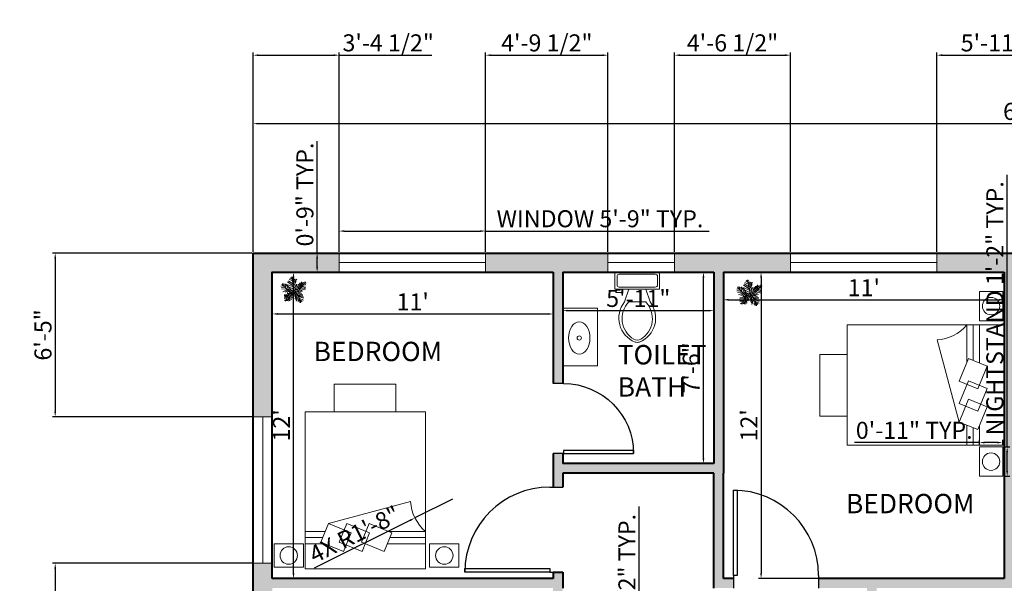
# Model space of a CAD drawing. Units: inches. Extents: x 529 to 1442, y 1029 to 1677.
# Tile 3 of 7: x 529 to 991, y 1412 to 1677. Entities that reach past the tile are written whole.
import ezdxf

# ---------------------------------------------------------------- set-up
doc = ezdxf.new("R2010")
doc.units = ezdxf.units.IN
for name, color, linetype, lineweight in [('A-ANNO-DIMS', 2, 'Continuous', 18), ('A-AREA-IDEN', 7, 'Continuous', 25), ('A-DOOR', 4, 'Continuous', 25), ('A-FLOR-FIXT', 9, 'Continuous', 18), ('A-FURN', 8, 'Continuous', 18), ('A-WALL-PATT', 252, 'Continuous', 13), ('tree', 70, 'Continuous', 13), ('wall', 7, 'Continuous', 40), ('window', 52, 'Continuous', 18)]:
    doc.layers.add(name, color=color, linetype=linetype, lineweight=lineweight)
doc.styles.get("Standard").update_dxf_attribs({"font": 'arial.ttf'})
doc.dimstyles.new('ISO-25', dxfattribs={"dimtxt": 8, "dimasz": 2.5, "dimexe": 1.25, "dimexo": 0.625, "dimtad": 1, "dimdec": 0, "dimlunit": 4, "dimtxsty": 'Standard', "dimcen": 2.5, "dimadec": 0, "dimazin": 0, "dimtfac": 1, "dimtdec": 0, "dimtmove": 0, "dimatfit": 3, "dimfxl": 1, "dimarcsym": 0})

# ---------------------------------------------------------------- blocks, each defined once
blk = doc.blocks.new('*U2')
for p, q in [((0, 0), (0, -6)), ((40, 0), (40, -6))]:
    blk.add_line(p, q)
blk.add_lwpolyline([(0, 0), (0, 40), (1.75, 40), (1.75, 0)], close=True)
blk.add_arc((0, 0), 40, 0, 90)
blk = doc.blocks.new('*U4')
for p, q in [((9.5, -6), (9.5, -2)), ((-10, -8.5), (-8, -8.5)), ((-10, -9.5), (-10, -8.5)), ((-8, -8.5), (-8, -8)), ((-7, -8), (-7, -9.5)), ((-4, -8), (-6, -14)), ((4, -8), (6, -14)), ((-7, -9.5), (-10, -9.5)), ((4, -14), (-4, -14))]:
    blk.add_line(p, q)
blk.add_lwpolyline([(10.5, -8), (10.5, 0), (-10.5, 0), (-10.5, -8)], close=True)
for points in [[(-9.5, -2), (-9.5, -6)], [(8.5, -1), (-8.5, -1)], [(-8.5, -7), (8.5, -7)]]:
    blk.add_lwpolyline(points)
for centre, radius, start, end in [((-8.62, -1.88), 0.884, 81.8699, 188.1301), ((8.62, -1.88), 0.884, 351.8699, 98.1301), ((-8.62, -6.12), 0.884, 171.8699, 278.1301), ((8.62, -6.12), 0.884, 261.8699, 8.1301), ((3.52, -21.58), 12.17, 141.4691, 247.9714), ((4.2, -21.82), 11.33, 136.3677, 238.9468), ((-3.52, -21.58), 12.17, 292.0284, 38.5307), ((-4.2, -21.82), 11.33, 301.053, 43.6321), ((0, -27.88), 4, 245.7318, 294.2682), ((0, -29), 4, 254.8605, 285.1395)]:
    blk.add_arc(centre, radius, start, end)
blk = doc.blocks.new('*U12')
for p, q in [((-7.288, 39.707), (-21.778, 46.673)), ((-8.737, 47.138), (-17.069, 52.711)), ((-10.186, 53.64), (-13.084, 55.962)), ((0, 0), (-10.5, 57)), ((-9.099, 51.782), (-6.563, 55.962)), ((-7.65, 43.423), (-2.578, 49.46)), ((-5.839, 35.992), (4.667, 48.067)), ((-5.114, 27.632), (10.463, 46.673)), ((-47.498, 19.737), (-55.83, 18.344)), ((-40.615, 13.7), (-55.105, 10.913)), ((-31.5, 4.5), (-52.5, 25.5)), ((-33.37, 6.269), (-52.207, 5.34)), ((-48.585, 21.131), (-49.309, 29.026)), ((-28.299, 3.483), (-47.86, -5.805)), ((-43.513, 28.561), (-42.427, 15.558)), ((-38.442, 26.239), (-34.819, 7.663)), ((-21.416, 3.018), (-38.079, -8.128)), ((-35.544, 28.097), (-24.314, 3.947)), ((0, 0), (-31.5, 4.5)), ((-14.533, 2.09), (-30.834, 25.31)), ((-15.982, 2.09), (-30.11, -9.521)), ((-3.665, 19.273), (-27.574, 35.527)), ((-5.114, 28.097), (-24.676, 40.636)), ((-24.314, 23.917), (-2.941, 13.7)), ((0, 0), (-22.5, -19.5)), ((-6.563, 1.161), (-21.416, -8.128)), ((-20.691, 13.7), (-1.129, 4.876)), ((-2.941, 16.486), (8.652, 37.85)), ((-1.129, 6.734), (9.014, 26.704)), ((0, 0), (27, 9)), ((0, 0), (18, -22.5)), ((3.942, 1.625), (11.187, 24.381)), ((6.478, 1.625), (26.04, -8.592)), ((10.101, 3.483), (17.708, 26.239)), ((11.187, 3.483), (30.749, -5.805)), ((16.259, 5.805), (23.142, 31.348)), ((18.07, 5.805), (35.096, -3.483)), ((22.055, 7.198), (27.489, 32.277)), ((24.229, 7.663), (46.688, 1.625)), ((27, 9), (48, 36)), ((27.127, 9.056), (31.112, 35.992)), ((29.662, 12.307), (48.137, 6.269)), ((31.836, 30.883), (32.561, 16.486)), ((33.285, 16.486), (48.862, 10.913)), ((35.096, 32.741), (37.27, 22.524)), ((36.183, 19.737), (48.137, 17.88)), ((38.719, 34.134), (41.979, 28.561)), ((40.53, 25.775), (48.862, 24.846)), ((43.791, 29.954), (51.036, 30.883)), ((44.153, 36.456), (45.239, 32.741)), ((-17.431, -15.094), (-42.789, -18.809)), ((-28.299, -29.026), (-42.789, -31.348)), ((-24.314, -21.596), (-42.427, -22.06)), ((-30.834, -34.135), (-42.427, -35.528)), ((-34.457, -39.708), (-40.978, -42.494)), ((-26.849, -26.24), (-40.253, -25.775)), ((-22.5, -19.5), (-37.5, -45)), ((-32.646, -36.921), (-31.921, -44.352)), ((-15.257, -12.772), (-30.11, -12.772)), ((-29.023, -30.884), (-27.936, -43.887)), ((-25.038, -23.918), (-22.865, -45.281)), ((-20.691, -18.345), (-17.793, -44.352)), ((-6.563, -5.805), (-19.967, -9.985)), ((-17.069, -15.094), (-12.721, -40.172)), ((-13.446, -11.378), (-8.737, -32.741)), ((-9.461, -8.592), (-6.201, -23.453)), ((-4.752, -3.483), (-3.665, -14.629)), ((2.493, -3.019), (-1.491, -20.202)), ((1.769, -2.555), (24.229, -9.521)), ((5.029, -6.27), (2.131, -25.775)), ((9.014, -11.378), (3.58, -35.992)), ((14.085, -16.951), (6.478, -40.172)), ((7.565, -9.056), (32.198, -14.629)), ((18.07, -22.524), (8.289, -45.745)), ((12.274, -15.094), (36.907, -18.809)), ((20.244, -30.419), (15.897, -44.816)), ((16.259, -19.738), (36.183, -22.989)), ((18, -22.5), (27, -52.5)), ((18.433, -22.524), (40.53, -29.026)), ((19.157, -25.311), (38.719, -33.206)), ((22.78, -37.85), (19.519, -48.532)), ((21.331, -32.741), (39.081, -40.636)), ((22.78, -38.314), (34.372, -44.816)), ((24.591, -45.745), (23.142, -50.854)), ((24.591, -43.423), (30.749, -47.603)), ((26.764, -49.925), (28.213, -50.854))]:
    blk.add_line(p, q)
blk = doc.blocks.new('*D13')
at = {"layer": 'A-ANNO-DIMS', "color": 0, "lineweight": -2, "transparency": 16777216}
for p, q in [((647.38, 1557.19), (647.38, 1536.93)), ((779.38, 1557.19), (779.38, 1536.93)), ((649.88, 1538.18), (776.88, 1538.18))]:
    blk.add_line(p, q, dxfattribs=at)
at = {"layer": 'A-ANNO-DIMS', "color": 0, "lineweight": 100, "transparency": 16777216}
for points in [[(649.88, 1538.6), (649.88, 1537.76), (647.38, 1538.18)], [(776.88, 1538.6), (776.88, 1537.76), (779.38, 1538.18)]]:
    blk.add_solid(points, dxfattribs=at)
at = {"layer": 'Defpoints', "color": 0, "lineweight": 100, "transparency": 16777216}
for p in [(647.38, 1557.81), (779.38, 1557.81), (779.38, 1538.18)]:
    blk.add_point(p, dxfattribs=at)
at = {"layer": 'A-ANNO-DIMS', "color": 0, "transparency": 16777216, "insert": (713.38, 1542.82), "char_height": 8, "attachment_point": 5}
blk.add_mtext("11'", dxfattribs=at)
blk = doc.blocks.new('*D14')
at = {"layer": 'A-ANNO-DIMS', "color": 0, "lineweight": -2, "transparency": 16777216}
for p, q in [((648.01, 1557.81), (658.61, 1557.81)), ((657.36, 1416.31), (657.36, 1555.31)), ((648.01, 1413.81), (658.61, 1413.81))]:
    blk.add_line(p, q, dxfattribs=at)
at = {"layer": 'A-ANNO-DIMS', "color": 0, "lineweight": 100, "transparency": 16777216}
for points in [[(656.94, 1555.31), (657.78, 1555.31), (657.36, 1557.81)], [(656.94, 1416.31), (657.78, 1416.31), (657.36, 1413.81)]]:
    blk.add_solid(points, dxfattribs=at)
at = {"layer": 'Defpoints', "color": 0, "lineweight": 100, "transparency": 16777216}
for p in [(647.38, 1557.81), (657.36, 1557.81), (647.38, 1413.81)]:
    blk.add_point(p, dxfattribs=at)
at = {"layer": 'A-ANNO-DIMS', "color": 0, "transparency": 16777216, "insert": (652.72, 1485.81), "char_height": 8, "attachment_point": 5, "rotation": 90}
blk.add_mtext("12'", dxfattribs=at)
blk = doc.blocks.new('*D15')
at = {"layer": 'A-ANNO-DIMS', "color": 0, "lineweight": -2, "transparency": 16777216}
for p, q in [((783.88, 1557.19), (783.88, 1538.48)), ((854.88, 1557.19), (854.88, 1538.48)), ((786.38, 1539.73), (852.38, 1539.73))]:
    blk.add_line(p, q, dxfattribs=at)
at = {"layer": 'A-ANNO-DIMS', "color": 0, "lineweight": 100, "transparency": 16777216}
for points in [[(786.38, 1540.15), (786.38, 1539.32), (783.88, 1539.73)], [(852.38, 1540.15), (852.38, 1539.32), (854.88, 1539.73)]]:
    blk.add_solid(points, dxfattribs=at)
at = {"layer": 'Defpoints', "color": 0, "lineweight": 100, "transparency": 16777216}
for p in [(783.88, 1557.81), (854.88, 1557.81), (854.88, 1539.73)]:
    blk.add_point(p, dxfattribs=at)
at = {"layer": 'A-ANNO-DIMS', "color": 0, "transparency": 16777216, "insert": (819.38, 1544.44), "char_height": 8, "attachment_point": 5}
blk.add_mtext('5\'-11"', dxfattribs=at)
blk = doc.blocks.new('*D16')
at = {"layer": 'A-ANNO-DIMS', "color": 0, "lineweight": -2, "transparency": 16777216}
for p, q in [((854.26, 1557.81), (848.76, 1557.81)), ((850.01, 1470.31), (850.01, 1555.31)), ((854.26, 1467.81), (848.76, 1467.81))]:
    blk.add_line(p, q, dxfattribs=at)
at = {"layer": 'A-ANNO-DIMS', "color": 0, "lineweight": 100, "transparency": 16777216}
for points in [[(849.59, 1555.31), (850.43, 1555.31), (850.01, 1557.81)], [(849.59, 1470.31), (850.43, 1470.31), (850.01, 1467.81)]]:
    blk.add_solid(points, dxfattribs=at)
at = {"layer": 'Defpoints', "color": 0, "lineweight": 100, "transparency": 16777216}
for p in [(850.01, 1557.81), (854.88, 1557.81), (854.88, 1467.81)]:
    blk.add_point(p, dxfattribs=at)
at = {"layer": 'A-ANNO-DIMS', "color": 0, "transparency": 16777216, "insert": (845.3, 1512.81), "char_height": 8, "attachment_point": 5, "rotation": 90}
blk.add_mtext('7\'-6"', dxfattribs=at)
blk = doc.blocks.new('*D17')
at = {"layer": 'A-ANNO-DIMS', "color": 0, "lineweight": -2, "transparency": 16777216}
for p, q in [((859.38, 1557.19), (859.38, 1543.59)), ((991.38, 1557.19), (991.38, 1543.59)), ((861.88, 1544.84), (988.88, 1544.84))]:
    blk.add_line(p, q, dxfattribs=at)
at = {"layer": 'A-ANNO-DIMS', "color": 0, "lineweight": 100, "transparency": 16777216}
for points in [[(861.88, 1545.26), (861.88, 1544.43), (859.38, 1544.84)], [(988.88, 1545.26), (988.88, 1544.43), (991.38, 1544.84)]]:
    blk.add_solid(points, dxfattribs=at)
at = {"layer": 'Defpoints', "color": 0, "lineweight": 100, "transparency": 16777216}
for p in [(859.38, 1557.81), (991.38, 1557.81), (991.38, 1544.84)]:
    blk.add_point(p, dxfattribs=at)
at = {"layer": 'A-ANNO-DIMS', "color": 0, "transparency": 16777216, "insert": (925.38, 1549.49), "char_height": 8, "attachment_point": 5}
blk.add_mtext("11'", dxfattribs=at)
blk = doc.blocks.new('*D18')
at = {"layer": 'A-ANNO-DIMS', "color": 0, "lineweight": -2, "transparency": 16777216}
for p, q in [((990.76, 1557.81), (875.84, 1557.81)), ((877.09, 1555.31), (877.09, 1416.31)), ((990.76, 1413.81), (875.84, 1413.81))]:
    blk.add_line(p, q, dxfattribs=at)
at = {"layer": 'A-ANNO-DIMS', "color": 0, "lineweight": 100, "transparency": 16777216}
for points in [[(876.67, 1555.31), (877.5, 1555.31), (877.09, 1557.81)], [(876.67, 1416.31), (877.5, 1416.31), (877.09, 1413.81)]]:
    blk.add_solid(points, dxfattribs=at)
at = {"layer": 'Defpoints', "color": 0, "lineweight": 100, "transparency": 16777216}
for p in [(991.38, 1557.81), (877.09, 1413.81), (991.38, 1413.81)]:
    blk.add_point(p, dxfattribs=at)
at = {"layer": 'A-ANNO-DIMS', "color": 0, "transparency": 16777216, "insert": (872.44, 1485.81), "char_height": 8, "attachment_point": 5, "rotation": 90}
blk.add_mtext("12'", dxfattribs=at)
blk = doc.blocks.new('*D55')
at = {"layer": 'A-ANNO-DIMS', "color": 0, "lineweight": -2, "transparency": 16777216}
for p, q in [((638.38, 1567.44), (638.38, 1628.88)), ((1358.38, 1567.44), (1358.38, 1628.88)), ((640.88, 1627.63), (1355.88, 1627.63))]:
    blk.add_line(p, q, dxfattribs=at)
at = {"layer": 'A-ANNO-DIMS', "color": 0, "lineweight": 100, "transparency": 16777216}
for points in [[(640.88, 1628.05), (640.88, 1627.22), (638.38, 1627.63)], [(1355.88, 1628.05), (1355.88, 1627.22), (1358.38, 1627.63)]]:
    blk.add_solid(points, dxfattribs=at)
at = {"layer": 'Defpoints', "color": 0, "lineweight": 100, "transparency": 16777216}
for p in [(1358.38, 1627.63), (638.38, 1566.81), (1358.38, 1566.81)]:
    blk.add_point(p, dxfattribs=at)
at = {"layer": 'A-ANNO-DIMS', "color": 0, "transparency": 16777216, "insert": (998.38, 1632.34), "char_height": 8, "attachment_point": 5}
blk.add_mtext("60'", dxfattribs=at)
blk = doc.blocks.new('WIN-LARGE-PLAN')
blk.add_line((0, 4.5), (68.85, 4.5))
blk.add_lwpolyline([(0, 9), (68.85, 9), (68.85, 0), (0, 0)], close=True)
blk = doc.blocks.new('WIN-SMALL-PLAN')
blk.add_line((0, 4.5), (31.29, 4.5))
blk.add_lwpolyline([(0, 9), (31.29, 9), (31.29, 0), (0, 0)], close=True)
blk = doc.blocks.new('BED-DOUBLE')
for p, q in [((10.82, 21.21), (49.46, 31.61)), ((0, 17.58), (9.33, 17.58)), ((0, 17.58), (9.33, 17.58)), ((0, 14.65), (8.12, 14.65)), ((28.37, 17.58), (28.47, 17.58)), ((28.37, 17.58), (28.47, 17.58)), ((38.76, 17.58), (56.44, 17.58)), ((38.76, 17.58), (56.44, 17.58)), ((39.74, 14.65), (56.44, 14.65)), ((0, 11.71), (9.09, 11.71)), ((28.13, 11.71), (28.23, 11.71)), ((38.53, 11.71), (56.44, 11.71))]:
    blk.add_line(p, q)
for points in [[(13.54, 73.79), (42.58, 73.79), (42.58, 86.74), (13.54, 86.74)], [(0, 0), (56.44, 0), (56.44, 73.79), (0, 73.79)], [(10.82, 21.21), (21.49, 16.82), (17.9, 8.09), (7.23, 12.48)], [(19.56, 21.21), (30.23, 16.82), (26.64, 8.09), (15.97, 12.48)], [(29.96, 21.21), (40.63, 16.82), (37.04, 8.09), (26.37, 12.48)]]:
    blk.add_lwpolyline(points, close=True)
blk.add_arc((69.23, 32.7), 19.8, 183.1428, 229.758)
blk = doc.blocks.new('NIGHTSTAND')
blk.add_lwpolyline([(0, 0), (13.77, 0), (13.77, 10.99), (0, 10.99)], close=True)
blk.add_circle((6.88, 5.5), 4.1)
blk = doc.blocks.new('WASHBASIN')
blk.add_lwpolyline([(0, 16.29), (27.02, 16.29), (27.02, 0), (0, 0)], close=True)
blk.add_circle((13.05, 8.54), 0.991)
blk.add_ellipse((13.05, 8.54), major_axis=(7.63, 0), ratio=0.659433)
blk = doc.blocks.new('*D71')
at = {"layer": 'A-ANNO-DIMS', "color": 0, "lineweight": -2, "transparency": 16777216}
for p, q in [((678.78, 1567.44), (678.78, 1578.39)), ((747.64, 1567.44), (747.64, 1578.39)), ((681.28, 1577.14), (745.14, 1577.14)), ((747.64, 1577.14), (852.62, 1577.14))]:
    blk.add_line(p, q, dxfattribs=at)
at = {"layer": 'A-ANNO-DIMS', "color": 0, "lineweight": 100, "transparency": 16777216}
for points in [[(681.28, 1577.56), (681.28, 1576.72), (678.78, 1577.14)], [(745.14, 1577.56), (745.14, 1576.72), (747.64, 1577.14)]]:
    blk.add_solid(points, dxfattribs=at)
at = {"layer": 'Defpoints', "color": 0, "lineweight": 100, "transparency": 16777216}
for p in [(747.64, 1577.14), (678.78, 1566.81), (747.64, 1566.81)]:
    blk.add_point(p, dxfattribs=at)
at = {"layer": 'A-ANNO-DIMS', "color": 0, "transparency": 16777216, "insert": (801.38, 1581.9), "char_height": 8, "attachment_point": 5}
blk.add_mtext('WINDOW 5\'-9" TYP.', dxfattribs=at)
blk = doc.blocks.new('*D72')
at = {"layer": 'A-ANNO-DIMS', "color": 0, "lineweight": -2, "transparency": 16777216}
for p, q in [((668.46, 1566.81), (668.46, 1619.33)), ((678.16, 1566.81), (667.21, 1566.81)), ((668.46, 1560.31), (668.46, 1564.31)), ((678.16, 1557.81), (667.21, 1557.81))]:
    blk.add_line(p, q, dxfattribs=at)
at = {"layer": 'A-ANNO-DIMS', "color": 0, "lineweight": 100, "transparency": 16777216}
for points in [[(668.04, 1564.31), (668.87, 1564.31), (668.46, 1566.81)], [(668.04, 1560.31), (668.87, 1560.31), (668.46, 1557.81)]]:
    blk.add_solid(points, dxfattribs=at)
at = {"layer": 'Defpoints', "color": 0, "lineweight": 100, "transparency": 16777216}
for p in [(668.46, 1566.81), (678.78, 1566.81), (678.78, 1557.81)]:
    blk.add_point(p, dxfattribs=at)
at = {"layer": 'A-ANNO-DIMS', "color": 0, "transparency": 16777216, "insert": (663.75, 1594.32), "char_height": 8, "attachment_point": 5, "rotation": 90}
blk.add_mtext('0\'-9" TYP.', dxfattribs=at)
blk = doc.blocks.new('*D79')
at = {"layer": 'A-ANNO-DIMS', "color": 0, "lineweight": -2, "transparency": 16777216}
for p, q in [((992.73, 1475.66), (992.73, 1603.54)), ((991.29, 1475.66), (993.98, 1475.66)), ((992.73, 1464.39), (992.73, 1473.16)), ((991.29, 1461.89), (993.98, 1461.89))]:
    blk.add_line(p, q, dxfattribs=at)
at = {"layer": 'A-ANNO-DIMS', "color": 0, "lineweight": 100, "transparency": 16777216}
for points in [[(992.31, 1473.16), (993.15, 1473.16), (992.73, 1475.66)], [(992.31, 1464.39), (993.15, 1464.39), (992.73, 1461.89)]]:
    blk.add_solid(points, dxfattribs=at)
at = {"layer": 'Defpoints', "color": 0, "lineweight": 100, "transparency": 16777216}
for p in [(990.66, 1475.66), (992.73, 1475.66), (990.66, 1461.89)]:
    blk.add_point(p, dxfattribs=at)
at = {"layer": 'A-ANNO-DIMS', "color": 0, "transparency": 16777216, "insert": (987.97, 1540.85), "char_height": 8, "attachment_point": 5, "rotation": 90}
blk.add_mtext('NIGHTSTAND 1\'-2" TYP.', dxfattribs=at)
blk = doc.blocks.new('*D80')
at = {"layer": 'A-ANNO-DIMS', "color": 0, "lineweight": -2, "transparency": 16777216}
for p, q in [((979.67, 1477.73), (920.94, 1477.73)), ((979.67, 1476.29), (979.67, 1478.98)), ((988.16, 1477.73), (982.17, 1477.73)), ((990.66, 1476.29), (990.66, 1478.98))]:
    blk.add_line(p, q, dxfattribs=at)
at = {"layer": 'A-ANNO-DIMS', "color": 0, "lineweight": 100, "transparency": 16777216}
for points in [[(982.17, 1478.14), (982.17, 1477.31), (979.67, 1477.73)], [(988.16, 1478.14), (988.16, 1477.31), (990.66, 1477.73)]]:
    blk.add_solid(points, dxfattribs=at)
at = {"layer": 'Defpoints', "color": 0, "lineweight": 100, "transparency": 16777216}
for p in [(979.67, 1477.73), (979.67, 1475.66), (990.66, 1475.66)]:
    blk.add_point(p, dxfattribs=at)
at = {"layer": 'A-ANNO-DIMS', "color": 0, "transparency": 16777216, "insert": (949.05, 1482.44), "char_height": 8, "attachment_point": 5}
blk.add_mtext('0\'-11" TYP.', dxfattribs=at)
blk = doc.blocks.new('*D81')
at = {"layer": 'A-ANNO-DIMS', "color": 0, "lineweight": -2, "transparency": 16777216}
for p, q in [((819.84, 1296.79), (819.84, 1447.64)), ((821.36, 1296.79), (818.59, 1296.79)), ((819.84, 1285), (819.84, 1294.29)), ((821.36, 1282.5), (818.59, 1282.5))]:
    blk.add_line(p, q, dxfattribs=at)
at = {"layer": 'A-ANNO-DIMS', "color": 0, "lineweight": 100, "transparency": 16777216}
for points in [[(819.43, 1294.29), (820.26, 1294.29), (819.84, 1296.79)], [(819.43, 1285), (820.26, 1285), (819.84, 1282.5)]]:
    blk.add_solid(points, dxfattribs=at)
at = {"layer": 'Defpoints', "color": 0, "lineweight": 100, "transparency": 16777216}
for p in [(819.84, 1296.79), (821.99, 1296.79), (821.99, 1282.5)]:
    blk.add_point(p, dxfattribs=at)
at = {"layer": 'A-ANNO-DIMS', "color": 0, "transparency": 16777216, "insert": (815.08, 1373.47), "char_height": 8, "attachment_point": 5, "rotation": 90}
blk.add_mtext('DINING CHAIR 1\'-2 1/2" TYP.', dxfattribs=at)
blk = doc.blocks.new('*D99')
at = {"layer": 'A-ANNO-DIMS', "color": 0, "lineweight": -2, "transparency": 16777216}
for p, q in [((638.38, 1567.44), (638.38, 1661.06)), ((678.78, 1567.44), (678.78, 1661.06)), ((640.88, 1659.81), (676.28, 1659.81)), ((678.78, 1659.81), (722.44, 1659.81))]:
    blk.add_line(p, q, dxfattribs=at)
at = {"layer": 'A-ANNO-DIMS', "color": 0, "lineweight": 100, "transparency": 16777216}
for points in [[(640.88, 1660.23), (640.88, 1659.4), (638.38, 1659.81)], [(676.28, 1660.23), (676.28, 1659.4), (678.78, 1659.81)]]:
    blk.add_solid(points, dxfattribs=at)
at = {"layer": 'Defpoints', "color": 0, "lineweight": 100, "transparency": 16777216}
for p in [(678.78, 1659.81), (638.38, 1566.81), (678.78, 1566.81)]:
    blk.add_point(p, dxfattribs=at)
at = {"layer": 'A-ANNO-DIMS', "color": 0, "transparency": 16777216, "insert": (701.86, 1664.58), "char_height": 8, "attachment_point": 5}
blk.add_mtext('3\'-4 1/2"', dxfattribs=at)
blk = doc.blocks.new('*D100')
at = {"layer": 'A-ANNO-DIMS', "color": 0, "lineweight": -2, "transparency": 16777216}
for p, q in [((747.64, 1567.44), (747.64, 1661.06)), ((805.14, 1567.44), (805.14, 1661.06)), ((750.14, 1659.81), (802.64, 1659.81))]:
    blk.add_line(p, q, dxfattribs=at)
at = {"layer": 'A-ANNO-DIMS', "color": 0, "lineweight": 100, "transparency": 16777216}
for points in [[(750.14, 1660.23), (750.14, 1659.4), (747.64, 1659.81)], [(802.64, 1660.23), (802.64, 1659.4), (805.14, 1659.81)]]:
    blk.add_solid(points, dxfattribs=at)
at = {"layer": 'Defpoints', "color": 0, "lineweight": 100, "transparency": 16777216}
for p in [(805.14, 1659.81), (747.64, 1566.81), (805.14, 1566.81)]:
    blk.add_point(p, dxfattribs=at)
at = {"layer": 'A-ANNO-DIMS', "color": 0, "transparency": 16777216, "insert": (776.39, 1664.57), "char_height": 8, "attachment_point": 5}
blk.add_mtext('4\'-9 1/2"', dxfattribs=at)
blk = doc.blocks.new('*D101')
at = {"layer": 'A-ANNO-DIMS', "color": 0, "lineweight": -2, "transparency": 16777216}
for p, q in [((836.43, 1567.44), (836.43, 1661.06)), ((890.86, 1567.44), (890.86, 1661.06)), ((838.93, 1659.81), (888.36, 1659.81))]:
    blk.add_line(p, q, dxfattribs=at)
at = {"layer": 'A-ANNO-DIMS', "color": 0, "lineweight": 100, "transparency": 16777216}
for points in [[(838.93, 1660.23), (838.93, 1659.4), (836.43, 1659.81)], [(888.36, 1660.23), (888.36, 1659.4), (890.86, 1659.81)]]:
    blk.add_solid(points, dxfattribs=at)
at = {"layer": 'Defpoints', "color": 0, "lineweight": 100, "transparency": 16777216}
for p in [(890.86, 1659.81), (836.43, 1566.81), (890.86, 1566.81)]:
    blk.add_point(p, dxfattribs=at)
at = {"layer": 'A-ANNO-DIMS', "color": 0, "transparency": 16777216, "insert": (863.65, 1664.57), "char_height": 8, "attachment_point": 5}
blk.add_mtext('4\'-6 1/2"', dxfattribs=at)
blk = doc.blocks.new('*D102')
at = {"layer": 'A-ANNO-DIMS', "color": 0, "lineweight": -2, "transparency": 16777216}
for p, q in [((959.72, 1567.44), (959.72, 1661.06)), ((1031.09, 1567.44), (1031.09, 1661.06)), ((962.22, 1659.81), (1028.59, 1659.81))]:
    blk.add_line(p, q, dxfattribs=at)
at = {"layer": 'A-ANNO-DIMS', "color": 0, "lineweight": 100, "transparency": 16777216}
for points in [[(962.22, 1660.23), (962.22, 1659.4), (959.72, 1659.81)], [(1028.59, 1660.23), (1028.59, 1659.4), (1031.09, 1659.81)]]:
    blk.add_solid(points, dxfattribs=at)
at = {"layer": 'Defpoints', "color": 0, "lineweight": 100, "transparency": 16777216}
for p in [(1031.09, 1659.81), (959.72, 1566.81), (1031.09, 1566.81)]:
    blk.add_point(p, dxfattribs=at)
at = {"layer": 'A-ANNO-DIMS', "color": 0, "transparency": 16777216, "insert": (995.41, 1664.57), "char_height": 8, "attachment_point": 5}
blk.add_mtext('5\'-11 1/2"', dxfattribs=at)
blk = doc.blocks.new('*D105')
at = {"layer": 'A-ANNO-DIMS', "color": 0, "lineweight": -2, "transparency": 16777216}
for p, q in [((637.76, 1566.81), (544.13, 1566.81)), ((545.38, 1564.31), (545.38, 1492.31)), ((637.76, 1489.81), (544.13, 1489.81))]:
    blk.add_line(p, q, dxfattribs=at)
at = {"layer": 'A-ANNO-DIMS', "color": 0, "lineweight": 100, "transparency": 16777216}
for points in [[(544.97, 1564.31), (545.8, 1564.31), (545.38, 1566.81)], [(544.97, 1492.31), (545.8, 1492.31), (545.38, 1489.81)]]:
    blk.add_solid(points, dxfattribs=at)
at = {"layer": 'Defpoints', "color": 0, "lineweight": 100, "transparency": 16777216}
for p in [(638.38, 1566.81), (545.38, 1489.81), (638.38, 1489.81)]:
    blk.add_point(p, dxfattribs=at)
at = {"layer": 'A-ANNO-DIMS', "color": 0, "transparency": 16777216, "insert": (540.67, 1528.31), "char_height": 8, "attachment_point": 5, "rotation": 90}
blk.add_mtext('6\'-5"', dxfattribs=at)
blk = doc.blocks.new('*D106')
at = {"layer": 'A-ANNO-DIMS', "color": 0, "lineweight": -2, "transparency": 16777216}
for p, q in [((637.76, 1420.96), (544.13, 1420.96)), ((545.38, 1418.46), (545.38, 1407.08)), ((637.76, 1404.58), (544.13, 1404.58)), ((545.38, 1404.58), (545.38, 1361.68))]:
    blk.add_line(p, q, dxfattribs=at)
at = {"layer": 'A-ANNO-DIMS', "color": 0, "lineweight": 100, "transparency": 16777216}
for points in [[(544.97, 1418.46), (545.8, 1418.46), (545.38, 1420.96)], [(544.97, 1407.08), (545.8, 1407.08), (545.38, 1404.58)]]:
    blk.add_solid(points, dxfattribs=at)
at = {"layer": 'Defpoints', "color": 0, "lineweight": 100, "transparency": 16777216}
for p in [(638.38, 1420.96), (545.38, 1404.58), (638.38, 1404.58)]:
    blk.add_point(p, dxfattribs=at)
at = {"layer": 'A-ANNO-DIMS', "color": 0, "transparency": 16777216, "insert": (540.62, 1381.88), "char_height": 8, "attachment_point": 5, "rotation": 90}
blk.add_mtext('1\'-4 1/2"', dxfattribs=at)
blk = doc.blocks.new('*D119')
at = {"layer": 'A-ANNO-DIMS', "color": 0, "lineweight": -2, "transparency": 16777216}
for p, q in [((732.15, 1451.11), (714.42, 1442.29)), ((667.25, 1418.83), (712.18, 1441.18))]:
    blk.add_line(p, q, dxfattribs=at)
at = {"layer": 'A-ANNO-DIMS', "color": 0, "lineweight": 100, "transparency": 16777216}
blk.add_solid([(712, 1441.55), (712.37, 1440.8), (714.42, 1442.29)], dxfattribs=at)
at = {"layer": 'Defpoints', "color": 0, "lineweight": 100, "transparency": 16777216}
for p in [(732.15, 1451.11), (714.42, 1442.29)]:
    blk.add_point(p, dxfattribs=at)
at = {"layer": 'A-ANNO-DIMS', "color": 0, "transparency": 16777216, "insert": (686.5, 1433.66), "char_height": 8, "attachment_point": 5, "rotation": 26.4493}
blk.add_mtext('4X R1\'-8"', dxfattribs=at)

msp = doc.modelspace()

# ---------------------------------------------------------------- hatches: boundary and pattern name
at = {"layer": 'A-WALL-PATT'}
h = msp.add_hatch(color=256, dxfattribs=at)
h.dxf.hatch_style = 1
h.paths.add_polyline_path([(678.78, 1566.81), (638.38, 1566.81), (638.38, 1489.81), (647.38, 1489.81), (647.38, 1557.81), (678.78, 1557.81)])
h.paths.add_polyline_path([(805.14, 1566.81), (747.64, 1566.81), (747.64, 1557.81), (779.38, 1557.81), (805.14, 1557.81)])
h.paths.add_polyline_path([(890.86, 1566.81), (836.43, 1566.81), (836.43, 1557.81), (854.88, 1557.81), (890.86, 1557.81)])
h.paths.add_polyline_path([(783.88, 1557.81), (779.38, 1557.81), (779.38, 1505.45), (783.88, 1505.45)])
h.paths.add_polyline_path([(783.88, 1472.6), (779.38, 1472.6), (779.38, 1456.82), (783.88, 1456.82)])
h.paths.add_polyline_path([(859.38, 1557.81), (854.88, 1557.81), (854.88, 1467.81), (783.88, 1467.81), (783.88, 1463.31), (859.38, 1463.31)])
h.paths.add_polyline_path([(859.38, 1463.31), (854.88, 1463.31), (854.88, 1409.31), (864.07, 1409.31), (864.07, 1413.81), (859.38, 1413.81)])
h.paths.add_polyline_path([(647.38, 1420.96), (638.38, 1420.96), (638.38, 1404.58), (647.38, 1404.58)])
h.paths.add_polyline_path([(779.38, 1413.81), (647.38, 1413.81), (647.38, 1409.31), (779.38, 1409.31)])
h.paths.add_polyline_path([(647.38, 1363.31), (647.38, 1375.08), (638.38, 1375.08), (638.38, 1330.97), (647.38, 1330.97)])
h.paths.add_polyline_path([(736.73, 1367.3, -0.004844), (736.74, 1367.81), (647.38, 1367.81), (647.38, 1363.31), (736.73, 1363.31)])
h.paths.add_polyline_path([(783.88, 1409.31), (779.38, 1409.31), (779.38, 1367.36), (770.88, 1367.36), (770.88, 1363.31), (783.88, 1363.31)])
h.paths.add_polyline_path([(770.88, 1367.36), (763.3, 1367.36), (763.3, 1367.3), (763.3, 1363.31), (766.38, 1363.31), (770.88, 1363.31)])
h.paths.add_polyline_path([(783.88, 1416.82), (779.38, 1416.82), (779.38, 1413.81), (779.38, 1409.31), (783.88, 1409.31)])
h.paths.add_polyline_path([(647.38, 1223.81), (647.38, 1262.11), (638.38, 1262.11), (638.38, 1146.81), (647.38, 1146.81), (647.38, 1155.81)])
h.paths.add_polyline_path([(659.49, 1228.31), (647.38, 1228.31), (647.38, 1223.81), (659.49, 1223.81)])
h.paths.add_polyline_path([(718.19, 1226.94), (718.19, 1228.31), (706.68, 1228.31), (706.68, 1223.81), (718.19, 1223.81)])
h.paths.add_polyline_path([(770.88, 1252.81), (786.93, 1252.81), (786.93, 1257.31), (770.88, 1257.31), (766.38, 1257.31), (766.38, 1228.31), (759.84, 1228.31), (759.84, 1226.94), (759.84, 1223.81), (766.38, 1223.81), (766.38, 1155.81), (770.88, 1155.81), (770.88, 1179.81)])
h.paths.add_polyline_path([(794.05, 1155.81), (766.38, 1155.81), (766.38, 1146.81), (794.05, 1146.81)])
h.paths.add_polyline_path([(859.38, 1155.81), (825.34, 1155.81), (825.34, 1146.81), (859.38, 1146.81)])
h = msp.add_hatch(color=256, dxfattribs=at)
h.dxf.hatch_style = 1
h.paths.add_polyline_path([(1031.09, 1566.81), (959.72, 1566.81), (959.72, 1557.81), (991.38, 1557.81), (1031.09, 1557.81)])
h.paths.add_polyline_path([(1000.38, 1557.81), (991.38, 1557.81), (991.38, 1413.81), (991.38, 1409.31), (1000.38, 1409.31)])
h.paths.add_polyline_path([(991.38, 1413.81), (904.07, 1413.81), (904.07, 1409.31), (991.38, 1409.31)])
h.paths.add_polyline_path([(931.38, 1409.31), (926.88, 1409.31), (926.88, 1359.54), (931.38, 1359.54)])
h.paths.add_polyline_path([(854.88, 1257.31), (835.24, 1257.31), (835.24, 1252.81), (854.36, 1252.81, -0.003534), (854.88, 1252.81)])
h.paths.add_polyline_path([(859.38, 1323.81), (991.38, 1323.81), (991.38, 1328.31), (931.38, 1328.31), (854.88, 1328.31), (854.88, 1155.81), (859.38, 1155.81)])
h.paths.add_polyline_path([(1000.38, 1323.81), (991.38, 1323.81), (991.38, 1155.81), (991.38, 1146.81), (1000.35, 1146.81), (1000.38, 1155.81)])
h.paths.add_polyline_path([(1041.38, 1328.31), (1000.38, 1328.31), (1000.38, 1323.81), (1041.38, 1323.81)])
h.paths.add_polyline_path([(1041.38, 1339.12), (1036.88, 1339.12), (1036.88, 1328.31), (1041.38, 1328.31)])
h.paths.add_polyline_path([(1000.38, 1328.31), (991.38, 1328.31), (991.38, 1323.81), (1000.38, 1323.81)])
h.paths.add_polyline_path([(1041.38, 1409.31), (1036.88, 1409.31), (1036.88, 1360.41), (1041.38, 1360.41)])
h.paths.add_polyline_path([(1042.64, 1413.81), (1000.38, 1413.81), (1000.38, 1409.31), (1042.64, 1409.31)])

# ---------------------------------------------------------------- linework, layer by layer
at = {"layer": 'wall'}
for p, q in [((638.38, 1566.81), (1358.38, 1566.81)), ((638.38, 1146.81), (638.38, 1566.81)), ((647.38, 1557.81), (779.38, 1557.81)), ((779.38, 1557.81), (779.38, 1505.45)), ((783.88, 1557.81), (783.88, 1505.45)), ((783.88, 1557.81), (854.88, 1557.81)), ((854.88, 1557.81), (854.88, 1467.81)), ((859.38, 1557.81), (859.38, 1463.31)), ((859.38, 1557.81), (991.38, 1557.81)), ((991.38, 1557.81), (991.38, 1413.81)), ((779.38, 1472.6), (779.38, 1456.82)), ((783.88, 1472.6), (783.88, 1467.81)), ((854.88, 1467.81), (783.88, 1467.81)), ((854.88, 1463.31), (783.88, 1463.31)), ((783.88, 1463.31), (783.88, 1456.82)), ((854.88, 1409.31), (854.88, 1463.31)), ((859.38, 1413.81), (859.38, 1463.31)), ((779.38, 1416.82), (779.38, 1413.81)), ((779.38, 1416.82), (783.88, 1416.82)), ((783.88, 1416.82), (783.88, 1409.31)), ((779.38, 1413.81), (647.38, 1413.81)), ((864.07, 1413.81), (859.38, 1413.81)), ((991.38, 1413.81), (904.07, 1413.81))]:
    msp.add_line(p, q, dxfattribs=at)
for points in [[(859.38, 1146.81), (638.38, 1146.81), (638.38, 1566.81), (1358.38, 1566.81), (1358.38, 1146.81), (1132.38, 1146.81)], [(647.38, 1413.81), (647.38, 1557.81), (779.38, 1557.81)], [(783.88, 1557.81), (854.88, 1557.81)], [(859.38, 1557.81), (991.38, 1557.81)]]:
    msp.add_lwpolyline(points, dxfattribs=at)

# ---------------------------------------------------------------- block references
at = {"layer": 'A-DOOR', "xscale": -0.8213486723457876, "yscale": 0.8213486723457876, "zscale": 0.8213486723457876, "rotation": 270}
msp.add_blockref('*U2', (784.31, 1472.6), dxfattribs=at)
at = {"layer": 'A-DOOR', "rotation": 90}
msp.add_blockref('*U2', (777.88, 1416.82), dxfattribs=at)
at = {"layer": 'A-DOOR'}
msp.add_blockref('*U2', (864.07, 1415.31), dxfattribs=at)
at = {"layer": 'A-FLOR-FIXT'}
msp.add_blockref('*U4', (818.89, 1557.81), dxfattribs=at)
at = {"layer": 'A-FLOR-FIXT', "rotation": 89.99999999999721}
msp.add_blockref('WASHBASIN', (800.18, 1513.84), dxfattribs=at)
at = {"layer": 'A-FURN'}
for name, p, rotation in [('NIGHTSTAND', (990.66, 1534.99), 89.9999999999987), ('BED-DOUBLE', (991.38, 1476.56), 90.0000000000004), ('NIGHTSTAND', (990.66, 1461.89), 89.99999999999706)]:
    msp.add_blockref(name, p, dxfattribs=dict(at, rotation=rotation))
for name, p in [('BED-DOUBLE', (662.92, 1418.41)), ('NIGHTSTAND', (648.25, 1419.13)), ('NIGHTSTAND', (721.34, 1419.13))]:
    msp.add_blockref(name, p, dxfattribs=at)
at = {"layer": 'tree', "xscale": 0.1116431773080361, "yscale": 0.1116431773080361, "zscale": 0.1116431773080361}
for p in [(657.69, 1549.27), (871.88, 1547.79)]:
    msp.add_blockref('*U12', p, dxfattribs=at)
at = {"layer": 'window'}
for name, p in [('WIN-LARGE-PLAN', (678.78, 1557.81)), ('WIN-SMALL-PLAN', (805.14, 1557.81)), ('WIN-LARGE-PLAN', (890.87, 1557.81))]:
    msp.add_blockref(name, p, dxfattribs=at)
at = {"layer": 'window', "rotation": 269.9999999999995}
msp.add_blockref('WIN-LARGE-PLAN', (638.38, 1489.81), dxfattribs=at)

# ---------------------------------------------------------------- texts
at = {"layer": 'A-AREA-IDEN', "char_height": 9.098, "attachment_point": 1}
for s, insert in [('BEDROOM', (666.82, 1525.1)), ('TOILET\\PBATH', (809.71, 1523.58)), ('BEDROOM', (916.97, 1453.59))]:
    msp.add_mtext_dynamic_manual_height_columns(s, width=307.5887, gutter_width=45.49, heights=[0], dxfattribs=dict(at, insert=insert))

# ---------------------------------------------------------------- dimensions: what is measured, and where the dimension line sits
at = {"layer": 'A-ANNO-DIMS'}
for base, p1, p2, override, picture, middle in [((678.78, 1659.81), (638.38, 1566.81), (678.78, 1566.81), {"dimdec": 1, "dimlfac": 1, "dimrnd": 0, "dimzin": 1, "dimdsep": 46, "dimlunit": 4, "dimfrac": 2}, '*D99', (701.86, 1664.58)), ((805.14, 1659.81), (747.64, 1566.81), (805.14, 1566.81), {"dimdec": 1, "dimlfac": 1, "dimrnd": 0, "dimzin": 1, "dimdsep": 46, "dimlunit": 4, "dimfrac": 2}, '*D100', (776.39, 1664.57)), ((890.86, 1659.81), (836.43, 1566.81), (890.86, 1566.81), {"dimdec": 1, "dimlfac": 1, "dimrnd": 0, "dimzin": 1, "dimdsep": 46, "dimlunit": 4, "dimfrac": 2}, '*D101', (863.65, 1664.57)), ((1031.09, 1659.81), (959.72, 1566.81), (1031.09, 1566.81), {"dimdec": 1, "dimlfac": 1, "dimrnd": 0, "dimzin": 1, "dimdsep": 46, "dimlunit": 4, "dimfrac": 2}, '*D102', (995.41, 1664.57)), ((1358.38, 1627.63), (638.38, 1566.81), (1358.38, 1566.81), {"dimclrd": 0, "dimclre": 0, "dimclrt": 0}, '*D55', (998.38, 1632.34)), ((779.38, 1538.18), (647.38, 1557.81), (779.38, 1557.81), {"dimclrd": 0, "dimclre": 0, "dimclrt": 0}, '*D13', (713.38, 1542.82)), ((854.88, 1539.73), (783.88, 1557.81), (854.88, 1557.81), {"dimclrd": 0, "dimclre": 0, "dimclrt": 0}, '*D15', (819.38, 1544.44)), ((991.38, 1544.84), (859.38, 1557.81), (991.38, 1557.81), {"dimclrd": 0, "dimclre": 0, "dimclrt": 0}, '*D17', (925.38, 1549.49))]:
    dim = msp.add_linear_dim(base=base, p1=p1, p2=p2, dimstyle='ISO-25', override=override, dxfattribs=at)
    dim.commit()
    dim.dimension.update_dxf_attribs({"geometry": picture, "text_midpoint": middle})
for base, p1, p2, angle, text, picture, middle in [((668.46, 1566.81), (678.78, 1557.81), (678.78, 1566.81), 90, '<> TYP.', '*D72', (663.75, 1594.32)), ((992.73, 1475.66), (990.66, 1461.89), (990.66, 1475.66), 90, 'NIGHTSTAND <> TYP.', '*D79', (987.97, 1540.85)), ((979.67, 1477.73), (990.66, 1475.66), (979.67, 1475.66), 180, '<> TYP.', '*D80', (949.05, 1482.44)), ((819.84, 1296.79), (821.99, 1282.5), (821.99, 1296.79), 90, 'DINING CHAIR <> TYP.', '*D81', (815.08, 1373.47))]:
    dim = msp.add_linear_dim(base=base, p1=p1, p2=p2, angle=angle, text=text, dimstyle='ISO-25', override={"dimdec": 1, "dimlfac": 1, "dimrnd": 0, "dimzin": 1, "dimdsep": 46, "dimlunit": 4, "dimfrac": 2}, dxfattribs=at)
    dim.commit()
    dim.dimension.update_dxf_attribs({"geometry": picture, "text_midpoint": middle})
dim = msp.add_linear_dim(base=(747.64, 1577.14), p1=(678.78, 1566.81), p2=(747.64, 1566.81), text='WINDOW <> TYP.', dimstyle='ISO-25', override={"dimdec": 1, "dimlfac": 1, "dimrnd": 0, "dimzin": 1, "dimdsep": 46, "dimlunit": 4, "dimfrac": 2}, dxfattribs=at)
dim.commit()
dim.dimension.update_dxf_attribs({"geometry": '*D71', "text_midpoint": (801.38, 1581.9)})
for base, p1, p2, override, picture, middle in [((545.38, 1489.81), (638.38, 1566.81), (638.38, 1489.81), {"dimdec": 1, "dimlfac": 1, "dimrnd": 0, "dimzin": 1, "dimdsep": 46, "dimlunit": 4, "dimfrac": 2}, '*D105', (540.67, 1528.31)), ((657.36, 1557.81), (647.38, 1413.81), (647.38, 1557.81), {"dimclrd": 0, "dimclre": 0, "dimclrt": 0}, '*D14', (652.72, 1485.81)), ((850.01, 1557.81), (854.88, 1467.81), (854.88, 1557.81), {"dimclrd": 0, "dimclre": 0, "dimclrt": 0}, '*D16', (845.3, 1512.81)), ((877.09, 1413.81), (991.38, 1557.81), (991.38, 1413.81), {"dimclrd": 0, "dimclre": 0, "dimclrt": 0}, '*D18', (872.44, 1485.81)), ((545.38, 1404.58), (638.38, 1420.96), (638.38, 1404.58), {"dimdec": 1, "dimlfac": 1, "dimrnd": 0, "dimzin": 1, "dimdsep": 46, "dimlunit": 4, "dimfrac": 2}, '*D106', (540.62, 1381.88))]:
    dim = msp.add_linear_dim(base=base, p1=p1, p2=p2, angle=90, dimstyle='ISO-25', override=override, dxfattribs=at)
    dim.commit()
    dim.dimension.update_dxf_attribs({"geometry": picture, "text_midpoint": middle})
dim = msp.add_radius_dim(center=(732.15, 1451.11), mpoint=(714.42, 1442.29), text='4X <>', dimstyle='ISO-25', override={"dimdec": 1, "dimlfac": 1, "dimrnd": 0, "dimzin": 1, "dimdsep": 46, "dimlunit": 4, "dimfrac": 2}, dxfattribs=at)
dim.commit()
dim.dimension.update_dxf_attribs({"geometry": '*D119', "text_midpoint": (686.5, 1433.66)})

doc.saveas('drawing.dxf')
